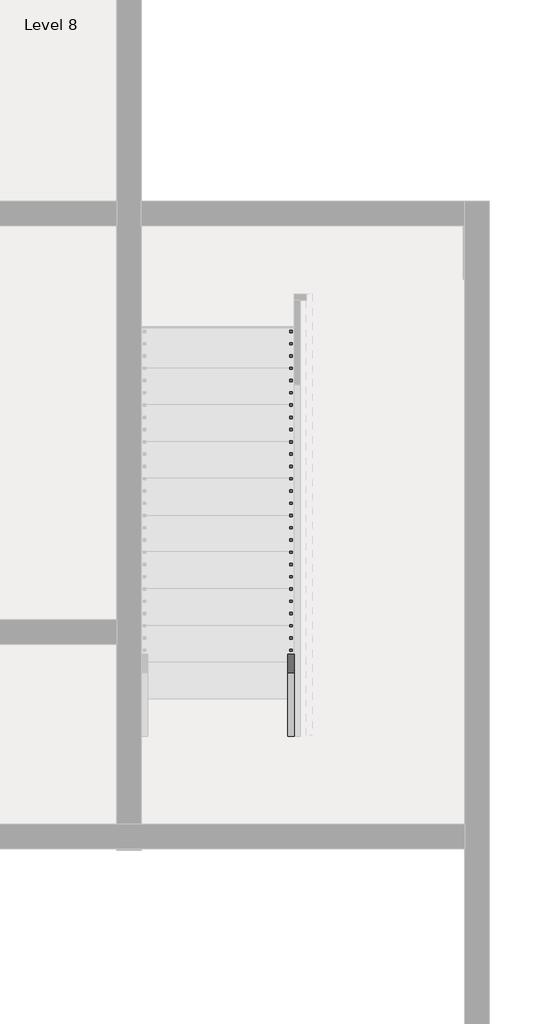
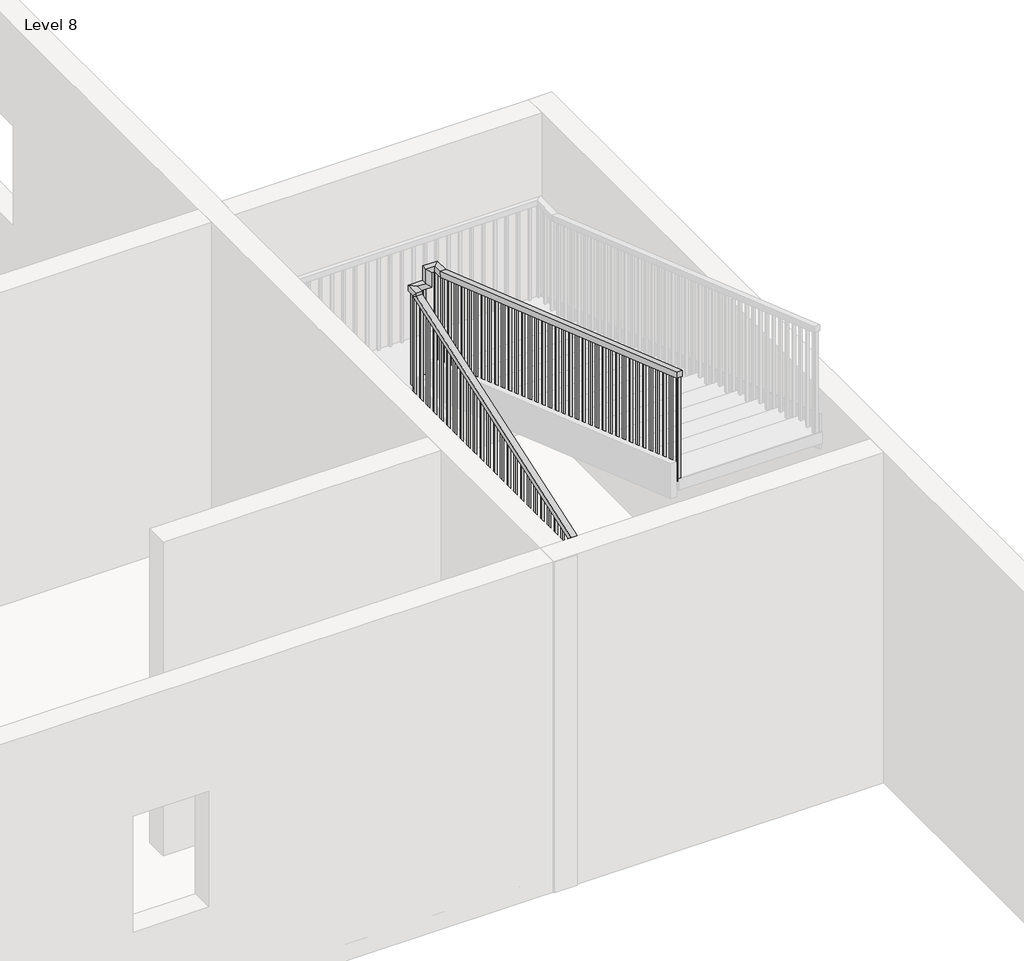
# One storey, part 6 of 14: 1 railing.
"""IFC4 building model written with IfcOpenShell, lengths in millimetres."""

from ifc_helpers import new_model, si_unit, frame, origin, place, context, project, spatial, polyline, outline, extrude, faceted_brep, element, save

model = new_model("IFC4")

# Units and contexts
model_context = context("Model", 3, world=origin())
ifc_project = project(units=[si_unit("LENGTHUNIT", "METRE", prefix="MILLI")], contexts=[model_context])

# Site, building, storey
site = spatial("IfcSite", under=ifc_project)
building = spatial("IfcBuilding", under=site)
storey = spatial("IfcBuildingStorey", under=building, Name="Level 8", Elevation=21336.0)

# Railing
placement = place(None, origin())
element("IfcRailing", 1, ObjectType="Handrail - Rectangular", at=placement, inside=storey, context=model_context, shape_type="SolidModel", body=[
    faceted_brep([(-2644.5381751, -9955.5916506, 22355.9076923), (-2644.5381751, -9955.5916506, 22302.1602476), (-2593.7381751, -9955.5916506, 22302.1602476), (-2593.7381751, -9955.5916506, 22355.9076923), (-2644.5381751, -6367.8416506, 23595.6687908), (-2644.5381751, -6317.0416506, 23559.4754856), (-2593.7381751, -6317.0416506, 23559.4754856), (-2593.7381751, -6367.8416506, 23595.6687908), (-2644.5381751, -6367.8416506, 23622.0), (-2644.5381751, -6317.0416506, 23571.2), (-2593.7381751, -6317.0416506, 23571.2), (-2593.7381751, -6367.8416506, 23622.0), (-2644.5381751, -6240.8416506, 23622.0), (-2644.5381751, -6240.8416506, 23571.2), (-2593.7381751, -6291.6416506, 23571.2), (-2593.7381751, -6291.6416506, 23622.0), (-2517.5381751, -6240.8416506, 23622.0), (-2466.7381751, -6240.8416506, 23571.2), (-2466.7381751, -6291.6416506, 23571.2), (-2517.5381751, -6291.6416506, 23622.0), (-2517.5381751, -6240.8416506, 23753.8846154), (-2466.7381751, -6240.8416506, 23703.0846154), (-2466.7381751, -6291.6416506, 23703.0846154), (-2517.5381751, -6291.6416506, 23753.8846154), (-2390.5381751, -6240.8416506, 23753.8846154), (-2390.5381751, -6240.8416506, 23703.0846154), (-2441.3381751, -6291.6416506, 23703.0846154), (-2441.3381751, -6291.6416506, 23753.8846154), (-2390.5381751, -6367.8416506, 23753.8846154), (-2390.5381751, -6376.3852679, 23703.0846154), (-2441.3381751, -6376.3852679, 23703.0846154), (-2441.3381751, -6367.8416506, 23753.8846154), (-2390.5381751, -9949.2416506, 24993.6), (-2441.3381751, -9949.2416506, 24993.6), (-2441.3381751, -9949.2416506, 24939.842594), (-2390.5381751, -9949.2416506, 24939.842594)], [[[0, 1, 2, 3]], [[1, 0, 4, 5]], [[2, 1, 5, 6]], [[3, 2, 6, 7]], [[0, 3, 7, 4]], [[5, 4, 8, 9]], [[6, 5, 9, 10]], [[7, 6, 10, 11]], [[4, 7, 11, 8]], [[9, 8, 12, 13]], [[10, 9, 13, 14]], [[11, 10, 14, 15]], [[8, 11, 15, 12]], [[13, 12, 16, 17]], [[14, 13, 17, 18]], [[15, 14, 18, 19]], [[12, 15, 19, 16]], [[17, 16, 20, 21]], [[18, 17, 21, 22]], [[19, 18, 22, 23]], [[16, 19, 23, 20]], [[21, 20, 24, 25]], [[22, 21, 25, 26]], [[23, 22, 26, 27]], [[20, 23, 27, 24]], [[25, 24, 28, 29]], [[26, 25, 29, 30]], [[27, 26, 30, 31]], [[24, 27, 31, 28]], [[32, 33, 34, 35]], [[29, 28, 32, 35]], [[30, 29, 35, 34]], [[31, 30, 34, 33]], [[28, 31, 33, 32]]]),
    extrude(outline(polyline([(-9933.3666506, 24934.3474017), (-9914.3166506, 24927.7531709), (-9914.3166506, 23973.6923077), (-9933.3666506, 23973.6923077), (-9933.3666506, 24934.3474017)])), frame((-2425.4631751, 0.0, 0.0), z_axis=(1.0, 0.0, 0.0), x_axis=(0.0, 1.0, 0.0)), (0.0, 0.0, 1.0), 19.05),
    extrude(outline(polyline([(-9831.7666506, 24899.1781709), (-9812.7166506, 24892.5839402), (-9812.7166506, 23973.6923077), (-9831.7666506, 23973.6923077), (-9831.7666506, 24899.1781709)])), frame((-2425.4631751, 0.0, 0.0), z_axis=(1.0, 0.0, 0.0), x_axis=(0.0, 1.0, 0.0)), (0.0, 0.0, 1.0), 19.05),
    extrude(outline(polyline([(-9730.1666506, 24864.0089402), (-9711.1166506, 24857.4147094), (-9711.1166506, 23973.6923077), (-9730.1666506, 23973.6923077), (-9730.1666506, 24864.0089402)])), frame((-2425.4631751, 0.0, 0.0), z_axis=(1.0, 0.0, 0.0), x_axis=(0.0, 1.0, 0.0)), (0.0, 0.0, 1.0), 19.05),
    extrude(outline(polyline([(-9628.5666506, 24828.8397094), (-9609.5166506, 24822.2454786), (-9609.5166506, 23868.1846154), (-9628.5666506, 23868.1846154), (-9628.5666506, 24828.8397094)])), frame((-2425.4631751, 0.0, 0.0), z_axis=(1.0, 0.0, 0.0), x_axis=(0.0, 1.0, 0.0)), (0.0, 0.0, 1.0), 19.05),
    extrude(outline(polyline([(-9526.9666506, 24793.6704786), (-9507.9166506, 24787.0762479), (-9507.9166506, 23868.1846154), (-9526.9666506, 23868.1846154), (-9526.9666506, 24793.6704786)])), frame((-2425.4631751, 0.0, 0.0), z_axis=(1.0, 0.0, 0.0), x_axis=(0.0, 1.0, 0.0)), (0.0, 0.0, 1.0), 19.05),
    extrude(outline(polyline([(-9425.3666506, 24758.5012479), (-9406.3166506, 24751.9070171), (-9406.3166506, 23868.1846154), (-9425.3666506, 23868.1846154), (-9425.3666506, 24758.5012479)])), frame((-2425.4631751, 0.0, 0.0), z_axis=(1.0, 0.0, 0.0), x_axis=(0.0, 1.0, 0.0)), (0.0, 0.0, 1.0), 19.05),
    extrude(outline(polyline([(-9323.7666506, 24723.3320171), (-9304.7166506, 24716.7377863), (-9304.7166506, 23762.6769231), (-9323.7666506, 23762.6769231), (-9323.7666506, 24723.3320171)])), frame((-2425.4631751, 0.0, 0.0), z_axis=(1.0, 0.0, 0.0), x_axis=(0.0, 1.0, 0.0)), (0.0, 0.0, 1.0), 19.05),
    extrude(outline(polyline([(-9222.1666506, 24688.1627863), (-9203.1166506, 24681.5685556), (-9203.1166506, 23762.6769231), (-9222.1666506, 23762.6769231), (-9222.1666506, 24688.1627863)])), frame((-2425.4631751, 0.0, 0.0), z_axis=(1.0, 0.0, 0.0), x_axis=(0.0, 1.0, 0.0)), (0.0, 0.0, 1.0), 19.05),
    extrude(outline(polyline([(-9120.5666506, 24652.9935556), (-9101.5166506, 24646.3993248), (-9101.5166506, 23762.6769231), (-9120.5666506, 23762.6769231), (-9120.5666506, 24652.9935556)])), frame((-2425.4631751, 0.0, 0.0), z_axis=(1.0, 0.0, 0.0), x_axis=(0.0, 1.0, 0.0)), (0.0, 0.0, 1.0), 19.05),
    extrude(outline(polyline([(-9018.9666506, 24617.8243248), (-8999.9166506, 24611.230094), (-8999.9166506, 23657.1692308), (-9018.9666506, 23657.1692308), (-9018.9666506, 24617.8243248)])), frame((-2425.4631751, 0.0, 0.0), z_axis=(1.0, 0.0, 0.0), x_axis=(0.0, 1.0, 0.0)), (0.0, 0.0, 1.0), 19.05),
    extrude(outline(polyline([(-8917.3666506, 24582.655094), (-8898.3166506, 24576.0608632), (-8898.3166506, 23657.1692308), (-8917.3666506, 23657.1692308), (-8917.3666506, 24582.655094)])), frame((-2425.4631751, 0.0, 0.0), z_axis=(1.0, 0.0, 0.0), x_axis=(0.0, 1.0, 0.0)), (0.0, 0.0, 1.0), 19.05),
    extrude(outline(polyline([(-8815.7666506, 24547.4858632), (-8796.7166506, 24540.8916325), (-8796.7166506, 23657.1692308), (-8815.7666506, 23657.1692308), (-8815.7666506, 24547.4858632)])), frame((-2425.4631751, 0.0, 0.0), z_axis=(1.0, 0.0, 0.0), x_axis=(0.0, 1.0, 0.0)), (0.0, 0.0, 1.0), 19.05),
    extrude(outline(polyline([(-8714.1666506, 24512.3166325), (-8695.1166506, 24505.7224017), (-8695.1166506, 23551.6615385), (-8714.1666506, 23551.6615385), (-8714.1666506, 24512.3166325)])), frame((-2425.4631751, 0.0, 0.0), z_axis=(1.0, 0.0, 0.0), x_axis=(0.0, 1.0, 0.0)), (0.0, 0.0, 1.0), 19.05),
    extrude(outline(polyline([(-8612.5666506, 24477.1474017), (-8593.5166506, 24470.5531709), (-8593.5166506, 23551.6615385), (-8612.5666506, 23551.6615385), (-8612.5666506, 24477.1474017)])), frame((-2425.4631751, 0.0, 0.0), z_axis=(1.0, 0.0, 0.0), x_axis=(0.0, 1.0, 0.0)), (0.0, 0.0, 1.0), 19.05),
    extrude(outline(polyline([(-8510.9666506, 24441.9781709), (-8491.9166506, 24435.3839402), (-8491.9166506, 23551.6615385), (-8510.9666506, 23551.6615385), (-8510.9666506, 24441.9781709)])), frame((-2425.4631751, 0.0, 0.0), z_axis=(1.0, 0.0, 0.0), x_axis=(0.0, 1.0, 0.0)), (0.0, 0.0, 1.0), 19.05),
    extrude(outline(polyline([(-8409.3666506, 24406.8089402), (-8390.3166506, 24400.2147094), (-8390.3166506, 23446.1538462), (-8409.3666506, 23446.1538462), (-8409.3666506, 24406.8089402)])), frame((-2425.4631751, 0.0, 0.0), z_axis=(1.0, 0.0, 0.0), x_axis=(0.0, 1.0, 0.0)), (0.0, 0.0, 1.0), 19.05),
    extrude(outline(polyline([(-8307.7666506, 24371.6397094), (-8288.7166506, 24365.0454786), (-8288.7166506, 23446.1538462), (-8307.7666506, 23446.1538462), (-8307.7666506, 24371.6397094)])), frame((-2425.4631751, 0.0, 0.0), z_axis=(1.0, 0.0, 0.0), x_axis=(0.0, 1.0, 0.0)), (0.0, 0.0, 1.0), 19.05),
    extrude(outline(polyline([(-8206.1666506, 24336.4704786), (-8187.1166506, 24329.8762479), (-8187.1166506, 23446.1538462), (-8206.1666506, 23446.1538462), (-8206.1666506, 24336.4704786)])), frame((-2425.4631751, 0.0, 0.0), z_axis=(1.0, 0.0, 0.0), x_axis=(0.0, 1.0, 0.0)), (0.0, 0.0, 1.0), 19.05),
    extrude(outline(polyline([(-8104.5666506, 24301.3012479), (-8085.5166506, 24294.7070171), (-8085.5166506, 23340.6461538), (-8104.5666506, 23340.6461538), (-8104.5666506, 24301.3012479)])), frame((-2425.4631751, 0.0, 0.0), z_axis=(1.0, 0.0, 0.0), x_axis=(0.0, 1.0, 0.0)), (0.0, 0.0, 1.0), 19.05),
    extrude(outline(polyline([(-8002.9666506, 24266.1320171), (-7983.9166506, 24259.5377863), (-7983.9166506, 23340.6461538), (-8002.9666506, 23340.6461538), (-8002.9666506, 24266.1320171)])), frame((-2425.4631751, 0.0, 0.0), z_axis=(1.0, 0.0, 0.0), x_axis=(0.0, 1.0, 0.0)), (0.0, 0.0, 1.0), 19.05),
    extrude(outline(polyline([(-7901.3666506, 24230.9627863), (-7882.3166506, 24224.3685556), (-7882.3166506, 23340.6461538), (-7901.3666506, 23340.6461538), (-7901.3666506, 24230.9627863)])), frame((-2425.4631751, 0.0, 0.0), z_axis=(1.0, 0.0, 0.0), x_axis=(0.0, 1.0, 0.0)), (0.0, 0.0, 1.0), 19.05),
    extrude(outline(polyline([(-7799.7666506, 24195.7935556), (-7780.7166506, 24189.1993248), (-7780.7166506, 23235.1384615), (-7799.7666506, 23235.1384615), (-7799.7666506, 24195.7935556)])), frame((-2425.4631751, 0.0, 0.0), z_axis=(1.0, 0.0, 0.0), x_axis=(0.0, 1.0, 0.0)), (0.0, 0.0, 1.0), 19.05),
    extrude(outline(polyline([(-7698.1666506, 24160.6243248), (-7679.1166506, 24154.030094), (-7679.1166506, 23235.1384615), (-7698.1666506, 23235.1384615), (-7698.1666506, 24160.6243248)])), frame((-2425.4631751, 0.0, 0.0), z_axis=(1.0, 0.0, 0.0), x_axis=(0.0, 1.0, 0.0)), (0.0, 0.0, 1.0), 19.05),
    extrude(outline(polyline([(-7596.5666506, 24125.455094), (-7577.5166506, 24118.8608632), (-7577.5166506, 23235.1384615), (-7596.5666506, 23235.1384615), (-7596.5666506, 24125.455094)])), frame((-2425.4631751, 0.0, 0.0), z_axis=(1.0, 0.0, 0.0), x_axis=(0.0, 1.0, 0.0)), (0.0, 0.0, 1.0), 19.05),
    extrude(outline(polyline([(-7494.9666506, 24090.2858632), (-7475.9166506, 24083.6916325), (-7475.9166506, 23129.6307692), (-7494.9666506, 23129.6307692), (-7494.9666506, 24090.2858632)])), frame((-2425.4631751, 0.0, 0.0), z_axis=(1.0, 0.0, 0.0), x_axis=(0.0, 1.0, 0.0)), (0.0, 0.0, 1.0), 19.05),
    extrude(outline(polyline([(-7393.3666506, 24055.1166325), (-7374.3166506, 24048.5224017), (-7374.3166506, 23129.6307692), (-7393.3666506, 23129.6307692), (-7393.3666506, 24055.1166325)])), frame((-2425.4631751, 0.0, 0.0), z_axis=(1.0, 0.0, 0.0), x_axis=(0.0, 1.0, 0.0)), (0.0, 0.0, 1.0), 19.05),
    extrude(outline(polyline([(-7291.7666506, 24019.9474017), (-7272.7166506, 24013.3531709), (-7272.7166506, 23129.6307692), (-7291.7666506, 23129.6307692), (-7291.7666506, 24019.9474017)])), frame((-2425.4631751, 0.0, 0.0), z_axis=(1.0, 0.0, 0.0), x_axis=(0.0, 1.0, 0.0)), (0.0, 0.0, 1.0), 19.05),
    extrude(outline(polyline([(-7190.1666506, 23984.7781709), (-7171.1166506, 23978.1839402), (-7171.1166506, 23024.1230769), (-7190.1666506, 23024.1230769), (-7190.1666506, 23984.7781709)])), frame((-2425.4631751, 0.0, 0.0), z_axis=(1.0, 0.0, 0.0), x_axis=(0.0, 1.0, 0.0)), (0.0, 0.0, 1.0), 19.05),
    extrude(outline(polyline([(-7088.5666506, 23949.6089402), (-7069.5166506, 23943.0147094), (-7069.5166506, 23024.1230769), (-7088.5666506, 23024.1230769), (-7088.5666506, 23949.6089402)])), frame((-2425.4631751, 0.0, 0.0), z_axis=(1.0, 0.0, 0.0), x_axis=(0.0, 1.0, 0.0)), (0.0, 0.0, 1.0), 19.05),
    extrude(outline(polyline([(-6986.9666506, 23914.4397094), (-6967.9166506, 23907.8454786), (-6967.9166506, 23024.1230769), (-6986.9666506, 23024.1230769), (-6986.9666506, 23914.4397094)])), frame((-2425.4631751, 0.0, 0.0), z_axis=(1.0, 0.0, 0.0), x_axis=(0.0, 1.0, 0.0)), (0.0, 0.0, 1.0), 19.05),
    extrude(outline(polyline([(-6885.3666506, 23879.2704786), (-6866.3166506, 23872.6762479), (-6866.3166506, 22918.6153846), (-6885.3666506, 22918.6153846), (-6885.3666506, 23879.2704786)])), frame((-2425.4631751, 0.0, 0.0), z_axis=(1.0, 0.0, 0.0), x_axis=(0.0, 1.0, 0.0)), (0.0, 0.0, 1.0), 19.05),
    extrude(outline(polyline([(-6783.7666506, 23844.1012479), (-6764.7166506, 23837.5070171), (-6764.7166506, 22918.6153846), (-6783.7666506, 22918.6153846), (-6783.7666506, 23844.1012479)])), frame((-2425.4631751, 0.0, 0.0), z_axis=(1.0, 0.0, 0.0), x_axis=(0.0, 1.0, 0.0)), (0.0, 0.0, 1.0), 19.05),
    extrude(outline(polyline([(-6682.1666506, 23808.9320171), (-6663.1166506, 23802.3377863), (-6663.1166506, 22918.6153846), (-6682.1666506, 22918.6153846), (-6682.1666506, 23808.9320171)])), frame((-2425.4631751, 0.0, 0.0), z_axis=(1.0, 0.0, 0.0), x_axis=(0.0, 1.0, 0.0)), (0.0, 0.0, 1.0), 19.05),
    extrude(outline(polyline([(-6580.5666506, 23773.7627863), (-6561.5166506, 23767.1685556), (-6561.5166506, 22813.1076923), (-6580.5666506, 22813.1076923), (-6580.5666506, 23773.7627863)])), frame((-2425.4631751, 0.0, 0.0), z_axis=(1.0, 0.0, 0.0), x_axis=(0.0, 1.0, 0.0)), (0.0, 0.0, 1.0), 19.05),
    extrude(outline(polyline([(-6478.9666506, 23738.5935556), (-6459.9166506, 23731.9993248), (-6459.9166506, 22813.1076923), (-6478.9666506, 22813.1076923), (-6478.9666506, 23738.5935556)])), frame((-2425.4631751, 0.0, 0.0), z_axis=(1.0, 0.0, 0.0), x_axis=(0.0, 1.0, 0.0)), (0.0, 0.0, 1.0), 19.05),
    extrude(outline(polyline([(-6377.3666506, 23703.4243248), (-6358.3166506, 23696.830094), (-6358.3166506, 22813.1076923), (-6377.3666506, 22813.1076923), (-6377.3666506, 23703.4243248)])), frame((-2425.4631751, 0.0, 0.0), z_axis=(1.0, 0.0, 0.0), x_axis=(0.0, 1.0, 0.0)), (0.0, 0.0, 1.0), 19.05),
    extrude(outline(polyline([(-2527.0631751, -6275.7666506), (-2527.0631751, -6256.7166506), (-2508.0131751, -6256.7166506), (-2508.0131751, -6275.7666506), (-2527.0631751, -6275.7666506)])), frame((0.0, 0.0, 22707.6), z_axis=(0.0, 0.0, 1.0), x_axis=(1.0, 0.0, 0.0)), (0.0, 0.0, 1.0), 863.6),
    extrude(outline(polyline([(-2609.6131751, -6307.5166506), (-2628.6631751, -6307.5166506), (-2628.6631751, -6288.4666506), (-2609.6131751, -6288.4666506), (-2609.6131751, -6307.5166506)])), frame((0.0, 0.0, 22602.0923077), z_axis=(0.0, 0.0, 1.0), x_axis=(1.0, 0.0, 0.0)), (0.0, 0.0, 1.0), 969.1076923),
    extrude(outline(polyline([(-6409.1166506, 23527.6586078), (-6390.0666506, 23534.2414101), (-6390.0666506, 22602.0923077), (-6409.1166506, 22602.0923077), (-6409.1166506, 23527.6586078)])), frame((-2628.6631751, 0.0, 0.0), z_axis=(1.0, 0.0, 0.0), x_axis=(0.0, 1.0, 0.0)), (0.0, 0.0, 1.0), 19.05),
    extrude(outline(polyline([(-6510.7166506, 23492.5503289), (-6491.6666506, 23499.1331312), (-6491.6666506, 22602.0923077), (-6510.7166506, 22602.0923077), (-6510.7166506, 23492.5503289)])), frame((-2628.6631751, 0.0, 0.0), z_axis=(1.0, 0.0, 0.0), x_axis=(0.0, 1.0, 0.0)), (0.0, 0.0, 1.0), 19.05),
    extrude(outline(polyline([(-6612.3166506, 23457.44205), (-6593.2666506, 23464.0248523), (-6593.2666506, 22496.5846154), (-6612.3166506, 22496.5846154), (-6612.3166506, 23457.44205)])), frame((-2628.6631751, 0.0, 0.0), z_axis=(1.0, 0.0, 0.0), x_axis=(0.0, 1.0, 0.0)), (0.0, 0.0, 1.0), 19.05),
    extrude(outline(polyline([(-6713.9166506, 23422.3337711), (-6694.8666506, 23428.9165734), (-6694.8666506, 22496.5846154), (-6713.9166506, 22496.5846154), (-6713.9166506, 23422.3337711)])), frame((-2628.6631751, 0.0, 0.0), z_axis=(1.0, 0.0, 0.0), x_axis=(0.0, 1.0, 0.0)), (0.0, 0.0, 1.0), 19.05),
    extrude(outline(polyline([(-6815.5166506, 23387.2254922), (-6796.4666506, 23393.8082945), (-6796.4666506, 22496.5846154), (-6815.5166506, 22496.5846154), (-6815.5166506, 23387.2254922)])), frame((-2628.6631751, 0.0, 0.0), z_axis=(1.0, 0.0, 0.0), x_axis=(0.0, 1.0, 0.0)), (0.0, 0.0, 1.0), 19.05),
    extrude(outline(polyline([(-6917.1166506, 23352.1172133), (-6898.0666506, 23358.7000156), (-6898.0666506, 22391.0769231), (-6917.1166506, 22391.0769231), (-6917.1166506, 23352.1172133)])), frame((-2628.6631751, 0.0, 0.0), z_axis=(1.0, 0.0, 0.0), x_axis=(0.0, 1.0, 0.0)), (0.0, 0.0, 1.0), 19.05),
    extrude(outline(polyline([(-7018.7166506, 23317.0089344), (-6999.6666506, 23323.5917367), (-6999.6666506, 22391.0769231), (-7018.7166506, 22391.0769231), (-7018.7166506, 23317.0089344)])), frame((-2628.6631751, 0.0, 0.0), z_axis=(1.0, 0.0, 0.0), x_axis=(0.0, 1.0, 0.0)), (0.0, 0.0, 1.0), 19.05),
    extrude(outline(polyline([(-7120.3166506, 23281.9006556), (-7101.2666506, 23288.4834578), (-7101.2666506, 22391.0769231), (-7120.3166506, 22391.0769231), (-7120.3166506, 23281.9006556)])), frame((-2628.6631751, 0.0, 0.0), z_axis=(1.0, 0.0, 0.0), x_axis=(0.0, 1.0, 0.0)), (0.0, 0.0, 1.0), 19.05),
    extrude(outline(polyline([(-7221.9166506, 23246.7923767), (-7202.8666506, 23253.375179), (-7202.8666506, 22285.5692308), (-7221.9166506, 22285.5692308), (-7221.9166506, 23246.7923767)])), frame((-2628.6631751, 0.0, 0.0), z_axis=(1.0, 0.0, 0.0), x_axis=(0.0, 1.0, 0.0)), (0.0, 0.0, 1.0), 19.05),
    extrude(outline(polyline([(-7323.5166506, 23211.6840978), (-7304.4666506, 23218.2669001), (-7304.4666506, 22285.5692308), (-7323.5166506, 22285.5692308), (-7323.5166506, 23211.6840978)])), frame((-2628.6631751, 0.0, 0.0), z_axis=(1.0, 0.0, 0.0), x_axis=(0.0, 1.0, 0.0)), (0.0, 0.0, 1.0), 19.05),
    extrude(outline(polyline([(-7425.1166506, 23176.5758189), (-7406.0666506, 23183.1586212), (-7406.0666506, 22285.5692308), (-7425.1166506, 22285.5692308), (-7425.1166506, 23176.5758189)])), frame((-2628.6631751, 0.0, 0.0), z_axis=(1.0, 0.0, 0.0), x_axis=(0.0, 1.0, 0.0)), (0.0, 0.0, 1.0), 19.05),
    extrude(outline(polyline([(-7526.7166506, 23141.46754), (-7507.6666506, 23148.0503423), (-7507.6666506, 22180.0615385), (-7526.7166506, 22180.0615385), (-7526.7166506, 23141.46754)])), frame((-2628.6631751, 0.0, 0.0), z_axis=(1.0, 0.0, 0.0), x_axis=(0.0, 1.0, 0.0)), (0.0, 0.0, 1.0), 19.05),
    extrude(outline(polyline([(-7628.3166506, 23106.3592611), (-7609.2666506, 23112.9420634), (-7609.2666506, 22180.0615385), (-7628.3166506, 22180.0615385), (-7628.3166506, 23106.3592611)])), frame((-2628.6631751, 0.0, 0.0), z_axis=(1.0, 0.0, 0.0), x_axis=(0.0, 1.0, 0.0)), (0.0, 0.0, 1.0), 19.05),
    extrude(outline(polyline([(-7729.9166506, 23071.2509822), (-7710.8666506, 23077.8337845), (-7710.8666506, 22180.0615385), (-7729.9166506, 22180.0615385), (-7729.9166506, 23071.2509822)])), frame((-2628.6631751, 0.0, 0.0), z_axis=(1.0, 0.0, 0.0), x_axis=(0.0, 1.0, 0.0)), (0.0, 0.0, 1.0), 19.05),
    extrude(outline(polyline([(-7831.5166506, 23036.1427033), (-7812.4666506, 23042.7255056), (-7812.4666506, 22074.5538462), (-7831.5166506, 22074.5538462), (-7831.5166506, 23036.1427033)])), frame((-2628.6631751, 0.0, 0.0), z_axis=(1.0, 0.0, 0.0), x_axis=(0.0, 1.0, 0.0)), (0.0, 0.0, 1.0), 19.05),
    extrude(outline(polyline([(-7933.1166506, 23001.0344244), (-7914.0666506, 23007.6172267), (-7914.0666506, 22074.5538462), (-7933.1166506, 22074.5538462), (-7933.1166506, 23001.0344244)])), frame((-2628.6631751, 0.0, 0.0), z_axis=(1.0, 0.0, 0.0), x_axis=(0.0, 1.0, 0.0)), (0.0, 0.0, 1.0), 19.05),
    extrude(outline(polyline([(-8034.7166506, 22965.9261455), (-8015.6666506, 22972.5089478), (-8015.6666506, 22074.5538462), (-8034.7166506, 22074.5538462), (-8034.7166506, 22965.9261455)])), frame((-2628.6631751, 0.0, 0.0), z_axis=(1.0, 0.0, 0.0), x_axis=(0.0, 1.0, 0.0)), (0.0, 0.0, 1.0), 19.05),
    extrude(outline(polyline([(-8136.3166506, 22930.8178666), (-8117.2666506, 22937.4006689), (-8117.2666506, 21969.0461538), (-8136.3166506, 21969.0461538), (-8136.3166506, 22930.8178666)])), frame((-2628.6631751, 0.0, 0.0), z_axis=(1.0, 0.0, 0.0), x_axis=(0.0, 1.0, 0.0)), (0.0, 0.0, 1.0), 19.05),
    extrude(outline(polyline([(-8237.9166506, 22895.7095877), (-8218.8666506, 22902.29239), (-8218.8666506, 21969.0461538), (-8237.9166506, 21969.0461538), (-8237.9166506, 22895.7095877)])), frame((-2628.6631751, 0.0, 0.0), z_axis=(1.0, 0.0, 0.0), x_axis=(0.0, 1.0, 0.0)), (0.0, 0.0, 1.0), 19.05),
    extrude(outline(polyline([(-8339.5166506, 22860.6013088), (-8320.4666506, 22867.1841111), (-8320.4666506, 21969.0461538), (-8339.5166506, 21969.0461538), (-8339.5166506, 22860.6013088)])), frame((-2628.6631751, 0.0, 0.0), z_axis=(1.0, 0.0, 0.0), x_axis=(0.0, 1.0, 0.0)), (0.0, 0.0, 1.0), 19.05),
    extrude(outline(polyline([(-8441.1166506, 22825.4930299), (-8422.0666506, 22832.0758322), (-8422.0666506, 21863.5384615), (-8441.1166506, 21863.5384615), (-8441.1166506, 22825.4930299)])), frame((-2628.6631751, 0.0, 0.0), z_axis=(1.0, 0.0, 0.0), x_axis=(0.0, 1.0, 0.0)), (0.0, 0.0, 1.0), 19.05),
    extrude(outline(polyline([(-8542.7166506, 22790.384751), (-8523.6666506, 22796.9675533), (-8523.6666506, 21863.5384615), (-8542.7166506, 21863.5384615), (-8542.7166506, 22790.384751)])), frame((-2628.6631751, 0.0, 0.0), z_axis=(1.0, 0.0, 0.0), x_axis=(0.0, 1.0, 0.0)), (0.0, 0.0, 1.0), 19.05),
    extrude(outline(polyline([(-8644.3166506, 22755.2764721), (-8625.2666506, 22761.8592744), (-8625.2666506, 21863.5384615), (-8644.3166506, 21863.5384615), (-8644.3166506, 22755.2764721)])), frame((-2628.6631751, 0.0, 0.0), z_axis=(1.0, 0.0, 0.0), x_axis=(0.0, 1.0, 0.0)), (0.0, 0.0, 1.0), 19.05),
    extrude(outline(polyline([(-8745.9166506, 22720.1681932), (-8726.8666506, 22726.7509955), (-8726.8666506, 21758.0307692), (-8745.9166506, 21758.0307692), (-8745.9166506, 22720.1681932)])), frame((-2628.6631751, 0.0, 0.0), z_axis=(1.0, 0.0, 0.0), x_axis=(0.0, 1.0, 0.0)), (0.0, 0.0, 1.0), 19.05),
    extrude(outline(polyline([(-8847.5166506, 22685.0599143), (-8828.4666506, 22691.6427166), (-8828.4666506, 21758.0307692), (-8847.5166506, 21758.0307692), (-8847.5166506, 22685.0599143)])), frame((-2628.6631751, 0.0, 0.0), z_axis=(1.0, 0.0, 0.0), x_axis=(0.0, 1.0, 0.0)), (0.0, 0.0, 1.0), 19.05),
    extrude(outline(polyline([(-8949.1166506, 22649.9516354), (-8930.0666506, 22656.5344377), (-8930.0666506, 21758.0307692), (-8949.1166506, 21758.0307692), (-8949.1166506, 22649.9516354)])), frame((-2628.6631751, 0.0, 0.0), z_axis=(1.0, 0.0, 0.0), x_axis=(0.0, 1.0, 0.0)), (0.0, 0.0, 1.0), 19.05),
    extrude(outline(polyline([(-9050.7166506, 22614.8433565), (-9031.6666506, 22621.4261588), (-9031.6666506, 21652.5230769), (-9050.7166506, 21652.5230769), (-9050.7166506, 22614.8433565)])), frame((-2628.6631751, 0.0, 0.0), z_axis=(1.0, 0.0, 0.0), x_axis=(0.0, 1.0, 0.0)), (0.0, 0.0, 1.0), 19.05),
    extrude(outline(polyline([(-9152.3166506, 22579.7350776), (-9133.2666506, 22586.3178799), (-9133.2666506, 21652.5230769), (-9152.3166506, 21652.5230769), (-9152.3166506, 22579.7350776)])), frame((-2628.6631751, 0.0, 0.0), z_axis=(1.0, 0.0, 0.0), x_axis=(0.0, 1.0, 0.0)), (0.0, 0.0, 1.0), 19.05),
    extrude(outline(polyline([(-9253.9166506, 22544.6267987), (-9234.8666506, 22551.209601), (-9234.8666506, 21652.5230769), (-9253.9166506, 21652.5230769), (-9253.9166506, 22544.6267987)])), frame((-2628.6631751, 0.0, 0.0), z_axis=(1.0, 0.0, 0.0), x_axis=(0.0, 1.0, 0.0)), (0.0, 0.0, 1.0), 19.05),
    extrude(outline(polyline([(-9355.5166506, 22509.5185198), (-9336.4666506, 22516.1013221), (-9336.4666506, 21547.0153846), (-9355.5166506, 21547.0153846), (-9355.5166506, 22509.5185198)])), frame((-2628.6631751, 0.0, 0.0), z_axis=(1.0, 0.0, 0.0), x_axis=(0.0, 1.0, 0.0)), (0.0, 0.0, 1.0), 19.05),
    extrude(outline(polyline([(-9457.1166506, 22474.4102409), (-9438.0666506, 22480.9930432), (-9438.0666506, 21547.0153846), (-9457.1166506, 21547.0153846), (-9457.1166506, 22474.4102409)])), frame((-2628.6631751, 0.0, 0.0), z_axis=(1.0, 0.0, 0.0), x_axis=(0.0, 1.0, 0.0)), (0.0, 0.0, 1.0), 19.05),
    extrude(outline(polyline([(-9558.7166506, 22439.301962), (-9539.6666506, 22445.8847643), (-9539.6666506, 21547.0153846), (-9558.7166506, 21547.0153846), (-9558.7166506, 22439.301962)])), frame((-2628.6631751, 0.0, 0.0), z_axis=(1.0, 0.0, 0.0), x_axis=(0.0, 1.0, 0.0)), (0.0, 0.0, 1.0), 19.05),
    extrude(outline(polyline([(-9660.3166506, 22404.1936831), (-9641.2666506, 22410.7764854), (-9641.2666506, 21441.5076923), (-9660.3166506, 21441.5076923), (-9660.3166506, 22404.1936831)])), frame((-2628.6631751, 0.0, 0.0), z_axis=(1.0, 0.0, 0.0), x_axis=(0.0, 1.0, 0.0)), (0.0, 0.0, 1.0), 19.05),
    extrude(outline(polyline([(-9761.9166506, 22369.0854043), (-9742.8666506, 22375.6682065), (-9742.8666506, 21441.5076923), (-9761.9166506, 21441.5076923), (-9761.9166506, 22369.0854043)])), frame((-2628.6631751, 0.0, 0.0), z_axis=(1.0, 0.0, 0.0), x_axis=(0.0, 1.0, 0.0)), (0.0, 0.0, 1.0), 19.05),
    extrude(outline(polyline([(-9863.5166506, 22333.9771254), (-9844.4666506, 22340.5599277), (-9844.4666506, 21441.5076923), (-9863.5166506, 21441.5076923), (-9863.5166506, 22333.9771254)])), frame((-2628.6631751, 0.0, 0.0), z_axis=(1.0, 0.0, 0.0), x_axis=(0.0, 1.0, 0.0)), (0.0, 0.0, 1.0), 19.05),
    extrude(outline(polyline([(-2425.4631751, -6275.7666506), (-2425.4631751, -6256.7166506), (-2406.4131751, -6256.7166506), (-2406.4131751, -6275.7666506), (-2425.4631751, -6275.7666506)])), frame((0.0, 0.0, 22707.6), z_axis=(0.0, 0.0, 1.0), x_axis=(1.0, 0.0, 0.0)), (0.0, 0.0, 1.0), 995.4846154),
    extrude(outline(polyline([(-2609.6131751, -6275.7666506), (-2628.6631751, -6275.7666506), (-2628.6631751, -6256.7166506), (-2609.6131751, -6256.7166506), (-2609.6131751, -6275.7666506)])), frame((0.0, 0.0, 22707.6), z_axis=(0.0, 0.0, 1.0), x_axis=(1.0, 0.0, 0.0)), (0.0, 0.0, 1.0), 863.6),
    extrude(outline(polyline([(-9949.2416506, 24939.842594), (-9930.1916506, 24933.2483632), (-9930.1916506, 23973.6923077), (-9949.2416506, 23973.6923077), (-9949.2416506, 24939.842594)])), frame((-2425.4631751, 0.0, 0.0), z_axis=(1.0, 0.0, 0.0), x_axis=(0.0, 1.0, 0.0)), (0.0, 0.0, 1.0), 19.05),
    extrude(outline(polyline([(-9955.5916506, 22302.1602476), (-9936.5416506, 22308.7430499), (-9936.5416506, 21441.5076923), (-9955.5916506, 21441.5076923), (-9955.5916506, 22302.1602476)])), frame((-2628.6631751, 0.0, 0.0), z_axis=(1.0, 0.0, 0.0), x_axis=(0.0, 1.0, 0.0)), (0.0, 0.0, 1.0), 19.05),
])

save(model, "model.ifc")

# Revit data of these elements
# Type "Handrail - Rectangular"
#   Assembly Code = "C2010400"
#   built-in parameter 1008612 = 0.0416667 (stored number, unit not read)
#   built-in parameter 1008611 = 0.0416667 (stored number, unit not read)
#   built-in parameter 1008609 = 0.333333 (stored number, unit not read)
#   built-in parameter 1008604 = 0.166667 (stored number, unit not read)
#   built-in parameter 1008603 = 0.166667 (stored number, unit not read)
#   Railing Height = 3' - 0"
#   built-in parameter 1008630 = 2
#   built-in parameter 1008610 = 2
#   built-in parameter 1008618 = Baluster - Square : 3/4"
# Element 1 (IfcRailing, "Handrail - Rectangular")
#   Phase Created = New Construction
